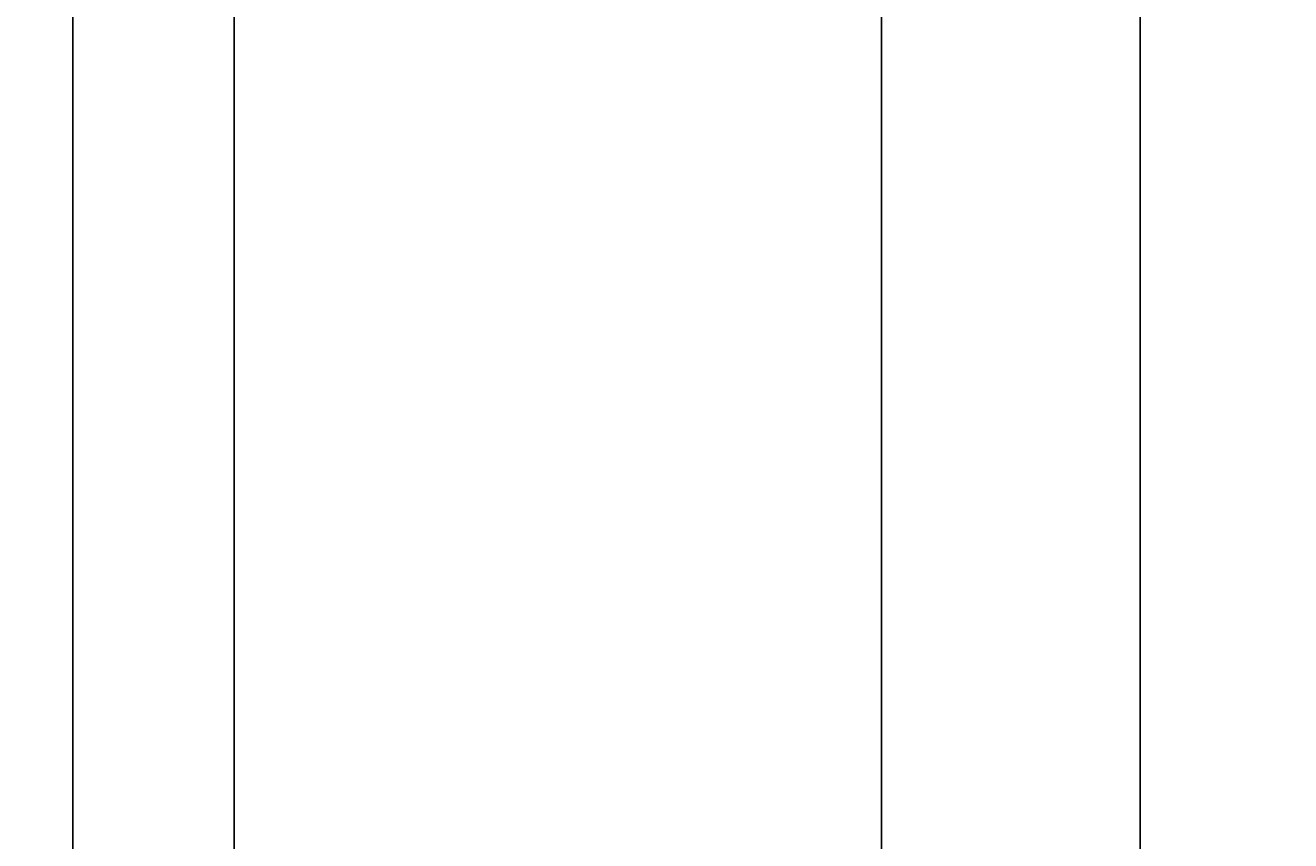
# Model space of a CAD drawing. Units: inches. Extents: x 738 to 1068, y 378 to 757.
# Tile 13 of 41: x 882 to 911, y 399 to 417. Entities that reach past the tile are written whole.
import ezdxf

# ---------------------------------------------------------------- set-up
doc = ezdxf.new("R2010")
doc.units = ezdxf.units.IN
doc.header["$MEASUREMENT"] = 0
doc.layers.add('A-ANNO-DIMS', color=2, linetype='Continuous', lineweight=18)
doc.styles.get("Standard").update_dxf_attribs({"font": 'arial.ttf'})
doc.dimstyles.get("Standard").update_dxf_attribs({"dimtxt": 0.18, "dimasz": 0.18, "dimexe": 0.18, "dimexo": 0.0625, "dimgap": 0.09, "dimtad": 0, "dimtih": 1, "dimtoh": 1, "dimdec": 4, "dimzin": 0, "dimdsep": 46, "dimtxsty": 'Standard', "dimcen": 0.09, "dimadec": 0, "dimazin": 0, "dimtfac": 1, "dimtdec": 4, "dimtofl": 0, "dimtmove": 0, "dimatfit": 3, "dimfxl": 1, "dimtolj": 1, "dimtzin": 0, "dimarcsym": 0})

# ---------------------------------------------------------------- blocks, each defined once
blk = doc.blocks.new('*D17')
at = {"layer": 'A-ANNO-DIMS', "color": 0, "lineweight": -2, "transparency": 16777216}
for p, q in [((1050.049, 415.919), (1050.049, 378.239)), ((756.324, 415.842), (756.324, 378.239)), ((756.504, 378.419), (902.791, 378.419)), ((1049.869, 378.419), (903.582, 378.419))]:
    blk.add_line(p, q, dxfattribs=at)
at = {"layer": 'A-ANNO-DIMS', "color": 0, "transparency": 16777216}
for points in [[(756.504, 378.449), (756.504, 378.389), (756.324, 378.419)], [(1049.869, 378.449), (1049.869, 378.389), (1050.049, 378.419)]]:
    blk.add_solid(points, dxfattribs=at)
at = {"layer": 'Defpoints', "color": 0, "transparency": 16777216}
for p in [(1050.049, 415.982), (756.324, 415.904), (1050.049, 378.419)]:
    blk.add_point(p, dxfattribs=at)
at = {"layer": 'A-ANNO-DIMS', "color": 0, "transparency": 16777216, "insert": (903.186, 378.419), "char_height": 0.18, "attachment_point": 5}
blk.add_mtext('\\A1;293.7', dxfattribs=at)
blk = doc.blocks.new('*D18')
at = {"layer": 'A-ANNO-DIMS', "color": 0, "lineweight": -2, "transparency": 16777216}
for p, q in [((901.525, 738.375), (1068.179, 738.375)), ((1067.999, 738.195), (1067.999, 569.167)), ((1067.999, 399.775), (1067.999, 568.803)), ((1023.842, 399.595), (1068.179, 399.595))]:
    blk.add_line(p, q, dxfattribs=at)
at = {"layer": 'A-ANNO-DIMS', "color": 0, "transparency": 16777216}
for points in [[(1067.969, 738.195), (1068.029, 738.195), (1067.999, 738.375)], [(1067.969, 399.775), (1068.029, 399.775), (1067.999, 399.595)]]:
    blk.add_solid(points, dxfattribs=at)
at = {"layer": 'Defpoints', "color": 0, "transparency": 16777216}
for p in [(901.462, 738.375), (1067.999, 738.375), (1023.779, 399.595)]:
    blk.add_point(p, dxfattribs=at)
at = {"layer": 'A-ANNO-DIMS', "color": 0, "transparency": 16777216, "insert": (1067.999, 568.985), "char_height": 0.18, "attachment_point": 5}
blk.add_mtext('\\A1;338.8', dxfattribs=at)
blk = doc.blocks.new('*D27')
at = {"layer": 'A-ANNO-DIMS', "color": 0, "lineweight": -2, "transparency": 16777216}
for p, q in [((883.457, 646.923), (883.457, 378.239)), ((923.511, 646.923), (923.511, 378.239)), ((883.637, 378.419), (903.086, 378.419)), ((923.331, 378.419), (903.882, 378.419))]:
    blk.add_line(p, q, dxfattribs=at)
at = {"layer": 'A-ANNO-DIMS', "color": 0, "transparency": 16777216}
for points in [[(883.637, 378.449), (883.637, 378.389), (883.457, 378.419)], [(923.331, 378.449), (923.331, 378.389), (923.511, 378.419)]]:
    blk.add_solid(points, dxfattribs=at)
at = {"layer": 'Defpoints', "color": 0, "transparency": 16777216}
for p in [(883.457, 646.985), (923.511, 646.985), (923.511, 378.419)]:
    blk.add_point(p, dxfattribs=at)
at = {"layer": 'A-ANNO-DIMS', "color": 0, "transparency": 16777216, "insert": (903.484, 378.419), "char_height": 0.18, "attachment_point": 5}
blk.add_mtext('\\A1;40.05', dxfattribs=at)
blk = doc.blocks.new('*D33')
at = {"layer": 'A-ANNO-DIMS', "color": 0, "lineweight": -2, "transparency": 16777216}
for p, q in [((836.324, 514.624), (836.324, 378.239)), ((907.171, 514.624), (907.171, 378.239)), ((836.504, 378.419), (871.354, 378.419)), ((906.991, 378.419), (872.141, 378.419))]:
    blk.add_line(p, q, dxfattribs=at)
at = {"layer": 'A-ANNO-DIMS', "color": 0, "transparency": 16777216}
for points in [[(836.504, 378.449), (836.504, 378.389), (836.324, 378.419)], [(906.991, 378.449), (906.991, 378.389), (907.171, 378.419)]]:
    blk.add_solid(points, dxfattribs=at)
at = {"layer": 'Defpoints', "color": 0, "transparency": 16777216}
for p in [(836.324, 514.687), (907.171, 514.687), (907.171, 378.419)]:
    blk.add_point(p, dxfattribs=at)
at = {"layer": 'A-ANNO-DIMS', "color": 0, "transparency": 16777216, "insert": (871.748, 378.419), "char_height": 0.18, "attachment_point": 5}
blk.add_mtext('\\A1;70.85', dxfattribs=at)
blk = doc.blocks.new('*D35')
at = {"layer": 'A-ANNO-DIMS', "color": 0, "lineweight": -2, "transparency": 16777216}
for p, q in [((855.932, 686.266), (855.932, 378.239)), ((901.429, 686.267), (901.429, 378.239)), ((856.112, 378.419), (878.352, 378.419)), ((901.249, 378.419), (879.009, 378.419))]:
    blk.add_line(p, q, dxfattribs=at)
at = {"layer": 'A-ANNO-DIMS', "color": 0, "transparency": 16777216}
for points in [[(856.112, 378.449), (856.112, 378.389), (855.932, 378.419)], [(901.249, 378.449), (901.249, 378.389), (901.429, 378.419)]]:
    blk.add_solid(points, dxfattribs=at)
at = {"layer": 'Defpoints', "color": 0, "transparency": 16777216}
for p in [(855.932, 686.329), (901.429, 686.329), (901.429, 378.419)]:
    blk.add_point(p, dxfattribs=at)
at = {"layer": 'A-ANNO-DIMS', "color": 0, "transparency": 16777216, "insert": (878.68, 378.419), "char_height": 0.18, "attachment_point": 5}
blk.add_mtext('\\A1;45.5', dxfattribs=at)
blk = doc.blocks.new('*D38')
at = {"layer": 'A-ANNO-DIMS', "color": 0, "lineweight": -2, "transparency": 16777216}
for p, q in [((781.485, 593.017), (781.485, 378.239)), ((887.04, 593.067), (887.04, 378.239)), ((781.665, 378.419), (833.807, 378.419)), ((886.86, 378.419), (834.718, 378.419))]:
    blk.add_line(p, q, dxfattribs=at)
at = {"layer": 'A-ANNO-DIMS', "color": 0, "transparency": 16777216}
for points in [[(781.665, 378.449), (781.665, 378.389), (781.485, 378.419)], [(886.86, 378.449), (886.86, 378.389), (887.04, 378.419)]]:
    blk.add_solid(points, dxfattribs=at)
at = {"layer": 'Defpoints', "color": 0, "transparency": 16777216}
for p in [(887.04, 593.13), (781.485, 593.08), (887.04, 378.419)]:
    blk.add_point(p, dxfattribs=at)
at = {"layer": 'A-ANNO-DIMS', "color": 0, "transparency": 16777216, "insert": (834.263, 378.419), "char_height": 0.18, "attachment_point": 5}
blk.add_mtext('\\A1;105.56', dxfattribs=at)
blk = doc.blocks.new('*D39')
at = {"layer": 'A-ANNO-DIMS', "color": 0, "lineweight": -2, "transparency": 16777216}
for p, q in [((887.04, 581.418), (887.04, 378.239)), ((938.455, 581.418), (938.455, 378.239)), ((887.22, 378.419), (912.371, 378.419)), ((938.275, 378.419), (913.124, 378.419))]:
    blk.add_line(p, q, dxfattribs=at)
at = {"layer": 'A-ANNO-DIMS', "color": 0, "transparency": 16777216}
for points in [[(887.22, 378.449), (887.22, 378.389), (887.04, 378.419)], [(938.275, 378.449), (938.275, 378.389), (938.455, 378.419)]]:
    blk.add_solid(points, dxfattribs=at)
at = {"layer": 'Defpoints', "color": 0, "transparency": 16777216}
for p in [(887.04, 581.481), (938.455, 581.481), (938.455, 378.419)]:
    blk.add_point(p, dxfattribs=at)
at = {"layer": 'A-ANNO-DIMS', "color": 0, "transparency": 16777216, "insert": (912.748, 378.419), "char_height": 0.18, "attachment_point": 5}
blk.add_mtext('\\A1;51.41', dxfattribs=at)

msp = doc.modelspace()

# ---------------------------------------------------------------- dimensions: what is measured, and where the dimension line sits
at = {"layer": 'A-ANNO-DIMS'}
dim = msp.add_linear_dim(base=(1067.9992, 738.3751), p1=(1023.779, 399.5952), p2=(901.4622, 738.3751), angle=90, dimstyle='Standard', override={"dimdec": 1, "dimlfac": 1, "dimrnd": 0, "dimzin": 0, "dimdsep": 46, "dimlunit": 2}, dxfattribs=at)
dim.commit()
dim.dimension.update_dxf_attribs({"geometry": '*D18', "text_midpoint": (1067.9992, 568.9851)})
for base, p1, p2, override, picture, middle in [((901.4286, 378.4191), (855.9323, 686.329), (901.4286, 686.3292), {"dimdec": 1, "dimlfac": 1, "dimrnd": 0, "dimzin": 0, "dimdsep": 46, "dimlunit": 2}, '*D35', (878.6804, 378.4191)), ((923.5105, 378.4191), (883.4574, 646.9853), (923.5105, 646.9853), {"dimdec": 2, "dimlfac": 1, "dimrnd": 0, "dimzin": 0, "dimdsep": 46, "dimlunit": 2}, '*D27', (903.484, 378.4191)), ((887.0404, 378.4191), (781.4846, 593.0796), (887.0404, 593.1296), {"dimdec": 2, "dimlfac": 1, "dimrnd": 0, "dimzin": 0, "dimdsep": 46, "dimlunit": 2}, '*D38', (834.2625, 378.4191)), ((938.455, 378.4191), (887.0404, 581.4808), (938.455, 581.4808), {"dimdec": 2, "dimlfac": 1, "dimrnd": 0, "dimzin": 0, "dimdsep": 46, "dimlunit": 2}, '*D39', (912.7477, 378.4191)), ((907.1708, 378.4191), (836.3244, 514.6866), (907.1708, 514.6866), {"dimdec": 2, "dimlfac": 1, "dimrnd": 0, "dimzin": 0, "dimdsep": 46, "dimlunit": 2}, '*D33', (871.7476, 378.4191)), ((1050.0492, 378.4191), (756.3236, 415.904), (1050.0492, 415.982), {"dimdec": 1, "dimlfac": 1, "dimrnd": 0, "dimzin": 0, "dimdsep": 46, "dimlunit": 2}, '*D17', (903.1864, 378.4191))]:
    dim = msp.add_linear_dim(base=base, p1=p1, p2=p2, dimstyle='Standard', override=override, dxfattribs=at)
    dim.commit()
    dim.dimension.update_dxf_attribs({"geometry": picture, "text_midpoint": middle})

doc.saveas('drawing.dxf')
